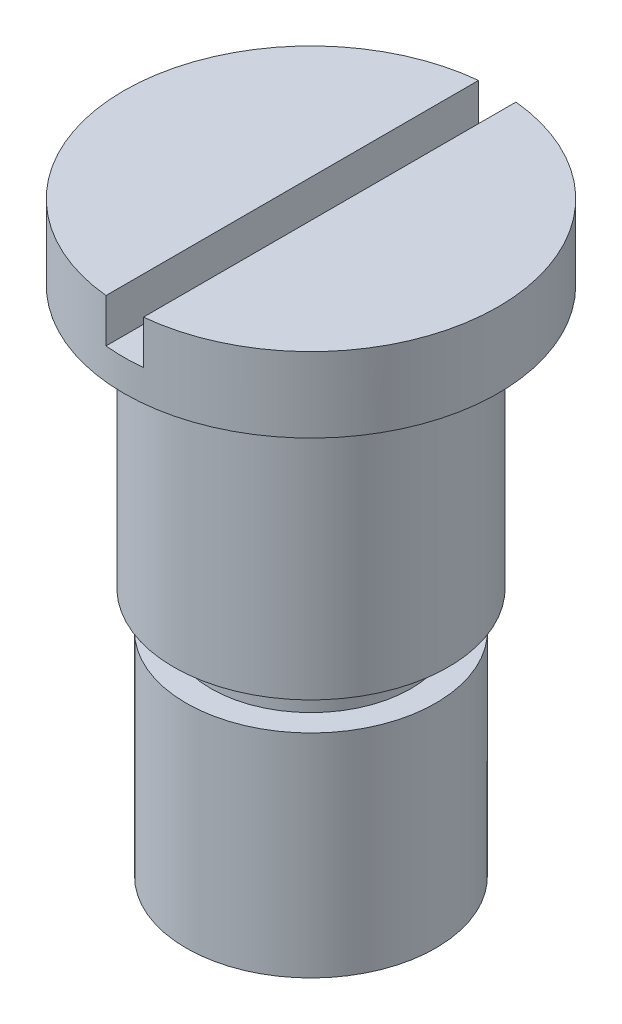
from build123d import *

# Parameters (mm, degrees)
LOWER_SHANK_SKETCH_20_R      = 10
LOWER_SHANK_20_DEPTH         = 17
GROOVE_NECK_SKETCH_16_R      = 8
GROOVE_NECK_16_DEPTH         = 3
UPPER_SHANK_SKETCH_22_R      = 11
UPPER_SHANK_22_DEPTH         = 21
HEAD_SKETCH_30_R             = 15
HEAD_30_DEPTH                = 6
SCREWDRIVER_SLOT_SKETCH_W    = 3
SCREWDRIVER_SLOT_SKETCH_H    = 32.46327366
SCREWDRIVER_SLOT_3X3_5_DEPTH = 3.5


with BuildPart() as part:
    # Lower Shank Sketch Ø20 → Lower Shank Ø20 (new body)
    with BuildSketch(Plane(origin=(0, 0, 0), x_dir=(1, 0, 0), z_dir=(0, 1, 0))):
        with Locations(Location((0, 0, 0), (0, 0, 270))):
            Circle(LOWER_SHANK_SKETCH_20_R)
    extrude(amount=LOWER_SHANK_20_DEPTH)

    # Groove Neck Sketch Ø16 → Groove Neck Ø16 (add)
    with BuildSketch(Plane(origin=(0, 17, 0), x_dir=(1, 0, 0), z_dir=(0, 1, 0))):
        with Locations(Location((0, 0, 0), (0, 0, 270))):
            Circle(GROOVE_NECK_SKETCH_16_R)
    extrude(amount=GROOVE_NECK_16_DEPTH)

    # Upper Shank Sketch Ø22 → Upper Shank Ø22 (add)
    with BuildSketch(Plane(origin=(0, 20, 0), x_dir=(1, 0, 0), z_dir=(0, 1, 0))):
        with Locations(Location((0, 0, 0), (0, 0, 90))):
            Circle(UPPER_SHANK_SKETCH_22_R)
    extrude(amount=UPPER_SHANK_22_DEPTH)

    # Head Sketch Ø30 → Head Ø30 (add)
    with BuildSketch(Plane(origin=(0, 41, 0), x_dir=(1, 0, 0), z_dir=(0, 1, 0))):
        with Locations(Location((0, 0, 0), (0, 0, 270))):
            Circle(HEAD_SKETCH_30_R)
    extrude(amount=HEAD_30_DEPTH)

    # Screwdriver Slot Sketch → Screwdriver Slot 3x3.5 (cut)
    with BuildSketch(Plane(origin=(0, 47, 0), x_dir=(1, 0, 0), z_dir=(0, 1, 0))):
        with Locations((0, -0.041354489)):
            Rectangle(SCREWDRIVER_SLOT_SKETCH_W, SCREWDRIVER_SLOT_SKETCH_H)
    extrude(amount=-SCREWDRIVER_SLOT_3X3_5_DEPTH, mode=Mode.SUBTRACT)


solid = part.part
